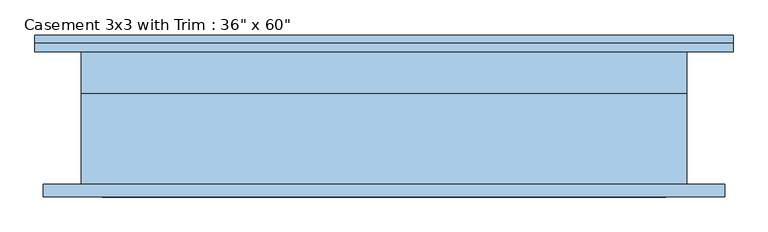
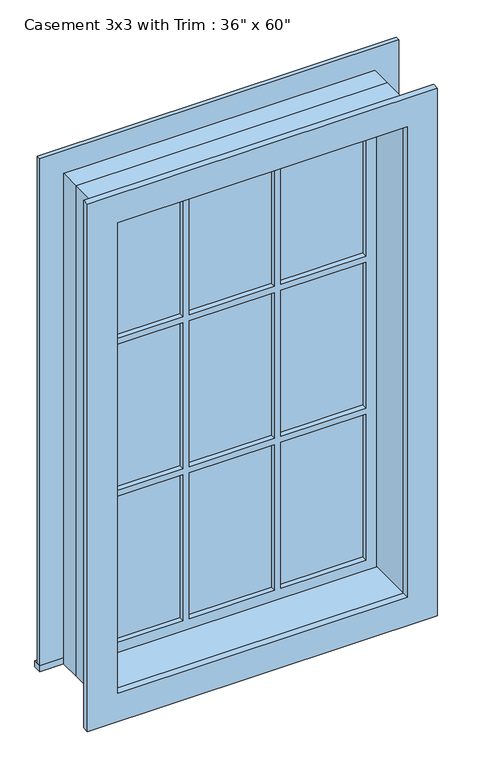
"""IFC4 building model written with IfcOpenShell, lengths in millimetres: window geometry."""

from ifc_helpers import new_model, si_unit, frame, origin, place, context, project, spatial, polyline, outline, extrude, source, transform, mapped, element, save


def window_3d3a5413(model_context):
    return source(origin(), model_context, "Body", "SweptSolid", [
        extrude(outline(polyline([(-527.05, 125.4), (527.05, 125.4), (527.05, 100.0), (-527.05, 100.0), (-527.05, 125.4)])), frame((0.0, 0.0, 609.6), z_axis=(0.0, 0.0, 1.0), x_axis=(1.0, 0.0, 0.0)), (0.0, 0.0, 1.0), 19.05),
        extrude(outline(polyline([(2114.55, -438.15), (2114.55, 438.15), (628.65, 438.15), (628.65, 527.05), (2203.45, 527.05), (2203.45, -527.05), (628.65, -527.05), (628.65, -438.15), (2114.55, -438.15)])), frame((0.0, 100.0, 0.0), z_axis=(0.0, 1.0, 0.0), x_axis=(0.0, 0.0, 1.0)), (0.0, 0.0, 1.0), 12.7),
        extrude(outline(polyline([(143.9333333, 65.075), (393.7, 65.075), (393.7, 52.375), (143.9333333, 52.375), (143.9333333, 65.075)])), frame((0.0, 0.0, 1617.1333333), z_axis=(0.0, 0.0, 1.0), x_axis=(1.0, 0.0, 0.0)), (0.0, 0.0, 1.0), 452.9666667),
        extrude(outline(polyline([(-124.8833333, 65.075), (124.8833333, 65.075), (124.8833333, 52.375), (-124.8833333, 52.375), (-124.8833333, 65.075)])), frame((0.0, 0.0, 1617.1333333), z_axis=(0.0, 0.0, 1.0), x_axis=(1.0, 0.0, 0.0)), (0.0, 0.0, 1.0), 452.9666667),
        extrude(outline(polyline([(-393.7, 65.075), (-143.9333333, 65.075), (-143.9333333, 52.375), (-393.7, 52.375), (-393.7, 65.075)])), frame((0.0, 0.0, 1617.1333333), z_axis=(0.0, 0.0, 1.0), x_axis=(1.0, 0.0, 0.0)), (0.0, 0.0, 1.0), 452.9666667),
        extrude(outline(polyline([(-393.7, 65.075), (-143.9333333, 65.075), (-143.9333333, 52.375), (-393.7, 52.375), (-393.7, 65.075)])), frame((0.0, 0.0, 1145.1166667), z_axis=(0.0, 0.0, 1.0), x_axis=(1.0, 0.0, 0.0)), (0.0, 0.0, 1.0), 452.9666667),
        extrude(outline(polyline([(-124.8833333, 65.075), (124.8833333, 65.075), (124.8833333, 52.375), (-124.8833333, 52.375), (-124.8833333, 65.075)])), frame((0.0, 0.0, 1145.1166667), z_axis=(0.0, 0.0, 1.0), x_axis=(1.0, 0.0, 0.0)), (0.0, 0.0, 1.0), 452.9666667),
        extrude(outline(polyline([(143.9333333, 65.075), (393.7, 65.075), (393.7, 52.375), (143.9333333, 52.375), (143.9333333, 65.075)])), frame((0.0, 0.0, 1145.1166667), z_axis=(0.0, 0.0, 1.0), x_axis=(1.0, 0.0, 0.0)), (0.0, 0.0, 1.0), 452.9666667),
        extrude(outline(polyline([(143.9333333, 65.075), (393.7, 65.075), (393.7, 52.375), (143.9333333, 52.375), (143.9333333, 65.075)])), frame((0.0, 0.0, 673.1), z_axis=(0.0, 0.0, 1.0), x_axis=(1.0, 0.0, 0.0)), (0.0, 0.0, 1.0), 452.9666667),
        extrude(outline(polyline([(-124.8833333, 65.075), (124.8833333, 65.075), (124.8833333, 52.375), (-124.8833333, 52.375), (-124.8833333, 65.075)])), frame((0.0, 0.0, 673.1), z_axis=(0.0, 0.0, 1.0), x_axis=(1.0, 0.0, 0.0)), (0.0, 0.0, 1.0), 452.9666667),
        extrude(outline(polyline([(-393.7, 65.075), (-143.9333333, 65.075), (-143.9333333, 52.375), (-393.7, 52.375), (-393.7, 65.075)])), frame((0.0, 0.0, 673.1), z_axis=(0.0, 0.0, 1.0), x_axis=(1.0, 0.0, 0.0)), (0.0, 0.0, 1.0), 452.9666667),
        extrude(outline(polyline([(2190.75, 514.35), (2190.75, -514.35), (552.45, -514.35), (552.45, 514.35), (2190.75, 514.35)]), holes=[polyline([(2101.85, 425.45), (641.35, 425.45), (641.35, -425.45), (2101.85, -425.45), (2101.85, 425.45)])]), frame((0.0, -119.05, 0.0), z_axis=(0.0, 1.0, 0.0), x_axis=(0.0, 0.0, 1.0)), (0.0, 0.0, 1.0), 19.05),
        extrude(outline(polyline([(2114.55, -438.15), (628.65, -438.15), (628.65, 438.15), (2114.55, 438.15), (2114.55, -438.15)]), holes=[polyline([(2070.1, -143.9333333), (1617.1333333, -143.9333333), (1617.1333333, -393.7), (2070.1, -393.7), (2070.1, -143.9333333)]), polyline([(1598.0833333, -143.9333333), (1145.1166667, -143.9333333), (1145.1166667, -393.7), (1598.0833333, -393.7), (1598.0833333, -143.9333333)]), polyline([(1126.0666667, -143.9333333), (673.1, -143.9333333), (673.1, -393.7), (1126.0666667, -393.7), (1126.0666667, -143.9333333)]), polyline([(2070.1, 124.8833333), (1617.1333333, 124.8833333), (1617.1333333, -124.8833333), (2070.1, -124.8833333), (2070.1, 124.8833333)]), polyline([(1598.0833333, 124.8833333), (1145.1166667, 124.8833333), (1145.1166667, -124.8833333), (1598.0833333, -124.8833333), (1598.0833333, 124.8833333)]), polyline([(1126.0666667, 124.8833333), (673.1, 124.8833333), (673.1, -124.8833333), (1126.0666667, -124.8833333), (1126.0666667, 124.8833333)]), polyline([(2070.1, 393.7), (1617.1333333, 393.7), (1617.1333333, 143.9333333), (2070.1, 143.9333333), (2070.1, 393.7)]), polyline([(1598.0833333, 393.7), (1145.1166667, 393.7), (1145.1166667, 143.9333333), (1598.0833333, 143.9333333), (1598.0833333, 393.7)]), polyline([(1126.0666667, 393.7), (673.1, 393.7), (673.1, 143.9333333), (1126.0666667, 143.9333333), (1126.0666667, 393.7)])]), frame((0.0, 36.5, 0.0), z_axis=(0.0, 1.0, 0.0), x_axis=(0.0, 0.0, 1.0)), (0.0, 0.0, 1.0), 44.45),
        extrude(outline(polyline([(2133.6, -457.2), (609.6, -457.2), (609.6, 457.2), (2133.6, 457.2), (2133.6, -457.2)]), holes=[polyline([(2101.85, -425.45), (2101.85, 425.45), (641.35, 425.45), (641.35, -425.45), (2101.85, -425.45)])]), frame((0.0, -100.0, 0.0), z_axis=(0.0, 1.0, 0.0), x_axis=(0.0, 0.0, 1.0)), (0.0, 0.0, 1.0), 136.5),
        extrude(outline(polyline([(2133.6, 457.2), (2133.6, -457.2), (609.6, -457.2), (609.6, 457.2), (2133.6, 457.2)]), holes=[polyline([(2114.55, 438.15), (628.65, 438.15), (628.65, -438.15), (2114.55, -438.15), (2114.55, 438.15)])]), frame((0.0, 36.5, 0.0), z_axis=(0.0, 1.0, 0.0), x_axis=(0.0, 0.0, 1.0)), (0.0, 0.0, 1.0), 63.5),
    ])


if __name__ == "__main__":
    model = new_model("IFC4")
    model_context = context("Model", 3, world=origin())
    ifc_project = project(units=[si_unit("LENGTHUNIT", "METRE", prefix="MILLI")], contexts=[model_context])
    site = spatial("IfcSite", under=ifc_project)
    building = spatial("IfcBuilding", under=site)
    placement = place(None, origin())
    window_shape = window_3d3a5413(model_context)
    element("IfcWindow", 1, ObjectType="Casement 3x3 with Trim : 36\" x 60\"", at=placement, inside=building, context=model_context, shape_type="MappedRepresentation", body=[
        mapped(window_shape, transform((0.0, 0.0, 0.0), x_axis=(1.0, 0.0, 0.0), y_axis=(0.0, 1.0, 0.0), z_axis=(0.0, 0.0, 1.0))),
    ])
    save(model, "model.ifc")

# Revit data of these elements
# Type "Casement 3x3 with Trim : 36\" x 60\""
#   Type Mark = "29"
#   Construction Type Id = "GSP4R"
#   Assembly Code = "B2020100"
#   Analytic Construction = "1/8 in Pilkington single glazing"
#   Visual Light Transmittance = 0.9
#   Solar Heat Gain Coefficient = 0.78
#   Heat Transfer Coefficient (U) = 3.6886 W/(m²·K)
#   Height = 5' - 0"
#   Default Sill Height = 2' - 0"
#   Trim Projection - Ext. = 0' - 0 1/2"
#   Trim Projection - Int. = 0' - 0 3/4"
#   Trim Width - Exterior = 0' - 3 1/2"
#   Trim Width - Interior = 0' - 3 1/2"
#   Width = 3' - 0"
#   Window Inset = 0' - 0 3/4"
#   Define Thermal Properties by = 1
#   Glass Pane Material = Glass
#   Sash Material = Sash
#   Trim Exterior Material = Trim
#   Trim Interior Material = Trim
#   Wall Closure = (empty or 0)
# Element 1 (IfcWindow, "Casement 3x3 with Trim : 36\" x 60\"")
#   Materials on its faces: "Sash", "Glass", "Trim"
# Materials
#   "Glass": class "Glass", colour RGB 218 227 224, transparency 0.85, Description = "Soda Lime Glass", Cost = 0
#   "Sash": class "Wood", colour RGB 136 99 55, transparency 0
#   "Trim": class "Wood", colour RGB 224 178 126, transparency 0
